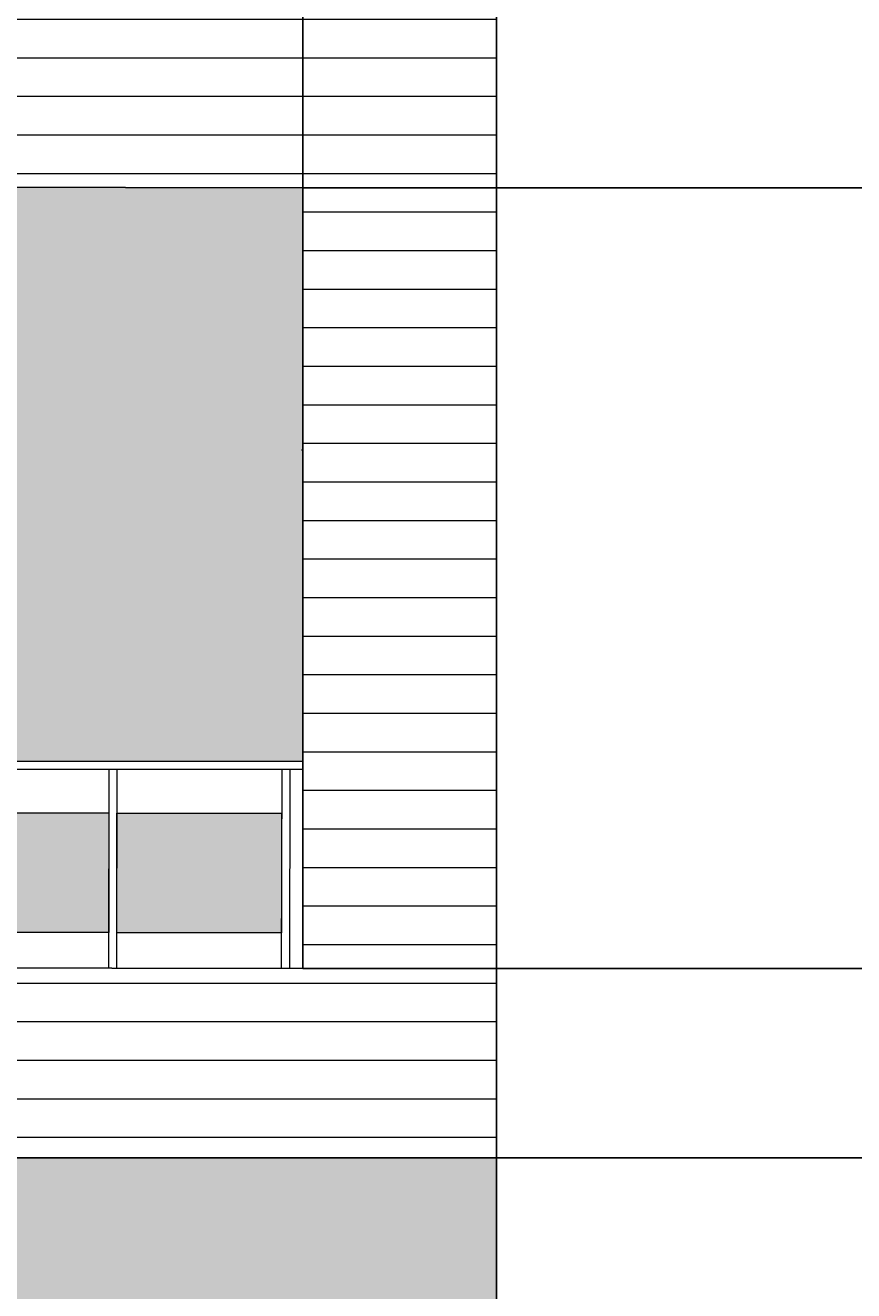
# Model space of a CAD drawing. Units: inches. Extents: x 36 to 594, y 79 to 831.
# Tile 14 of 30: x 390 to 492, y 290 to 446. Entities that reach past the tile are written whole.
import ezdxf

# ---------------------------------------------------------------- set-up
doc = ezdxf.new("R2010")
doc.units = ezdxf.units.IN
doc.header["$MEASUREMENT"] = 0
for name, color, linetype, lineweight in [('A-ANNO-DIMS', 2, 'Continuous', 18), ('A-ELEV', 7, 'Continuous', 25), ('A-ELEV-PATT', 8, 'Continuous', 13), ('A-GLAZ', 4, 'Continuous', 18)]:
    doc.layers.add(name, color=color, linetype=linetype, lineweight=lineweight)
doc.styles.get("Standard").update_dxf_attribs({"font": 'arial.ttf'})
doc.dimstyles.get("Standard").update_dxf_attribs({"dimtxt": 0.8125, "dimasz": 0.18, "dimexe": 0.18, "dimexo": 0.0625, "dimgap": 0.09, "dimtad": 0, "dimtih": 1, "dimtoh": 1, "dimdec": 4, "dimzin": 0, "dimdsep": 46, "dimlunit": 4, "dimtxsty": 'Standard', "dimcen": 0.09, "dimadec": 0, "dimazin": 0, "dimtfac": 1, "dimtdec": 4, "dimtofl": 0, "dimtmove": 0, "dimatfit": 3, "dimfxl": 1, "dimtolj": 1, "dimtzin": 0, "dimarcsym": 0})

# ---------------------------------------------------------------- blocks, each defined once
blk = doc.blocks.new('GLAZ-PANEL')
blk.add_lwpolyline([(0, 14.77), (20.28, 14.77), (20.28, 0), (0, 0)], close=True)
blk = doc.blocks.new('*D31')
at = {"layer": 'A-ANNO-DIMS', "color": 0, "lineweight": -2, "transparency": 16777216}
for p, q in [((448.45, 306.21), (592.85, 306.21)), ((592.67, 306.03), (592.67, 229.08)), ((592.67, 151.11), (592.67, 228.07)), ((401.61, 150.93), (592.85, 150.93))]:
    blk.add_line(p, q, dxfattribs=at)
at = {"layer": 'A-ANNO-DIMS', "color": 0, "transparency": 16777216}
for points in [[(592.64, 306.03), (592.7, 306.03), (592.67, 306.21)], [(592.64, 151.11), (592.7, 151.11), (592.67, 150.93)]]:
    blk.add_solid(points, dxfattribs=at)
at = {"layer": 'Defpoints', "color": 0, "transparency": 16777216}
for p in [(448.39, 306.21), (592.67, 306.21), (401.55, 150.93)]:
    blk.add_point(p, dxfattribs=at)
at = {"layer": 'A-ANNO-DIMS', "color": 0, "transparency": 16777216, "insert": (592.67, 228.57), "char_height": 0.812, "attachment_point": 5}
blk.add_mtext('\\A1;155.28', dxfattribs=at)
blk = doc.blocks.new('*D32')
at = {"layer": 'A-ANNO-DIMS', "color": 0, "lineweight": -2, "transparency": 16777216}
for p, q in [((424.61, 329.53), (592.85, 329.53)), ((592.67, 329.35), (592.67, 318.38)), ((592.67, 306.39), (592.67, 317.37)), ((448.45, 306.21), (592.85, 306.21))]:
    blk.add_line(p, q, dxfattribs=at)
at = {"layer": 'A-ANNO-DIMS', "color": 0, "transparency": 16777216}
for points in [[(592.64, 329.35), (592.7, 329.35), (592.67, 329.53)], [(592.64, 306.39), (592.7, 306.39), (592.67, 306.21)]]:
    blk.add_solid(points, dxfattribs=at)
at = {"layer": 'Defpoints', "color": 0, "transparency": 16777216}
for p in [(424.55, 329.53), (592.67, 329.53), (448.39, 306.21)]:
    blk.add_point(p, dxfattribs=at)
at = {"layer": 'A-ANNO-DIMS', "color": 0, "transparency": 16777216, "insert": (592.67, 317.87), "char_height": 0.812, "attachment_point": 5}
blk.add_mtext('\\A1;23.32', dxfattribs=at)
blk = doc.blocks.new('*D33')
at = {"layer": 'A-ANNO-DIMS', "color": 0, "lineweight": -2, "transparency": 16777216}
for p, q in [((424.61, 425.73), (592.85, 425.73)), ((592.67, 425.55), (592.67, 378.14)), ((592.67, 329.71), (592.67, 377.13)), ((424.61, 329.53), (592.85, 329.53))]:
    blk.add_line(p, q, dxfattribs=at)
at = {"layer": 'A-ANNO-DIMS', "color": 0, "transparency": 16777216}
for points in [[(592.64, 425.55), (592.7, 425.55), (592.67, 425.73)], [(592.64, 329.71), (592.7, 329.71), (592.67, 329.53)]]:
    blk.add_solid(points, dxfattribs=at)
at = {"layer": 'Defpoints', "color": 0, "transparency": 16777216}
for p in [(424.55, 425.73), (592.67, 425.73), (424.55, 329.53)]:
    blk.add_point(p, dxfattribs=at)
at = {"layer": 'A-ANNO-DIMS', "color": 0, "transparency": 16777216, "insert": (592.67, 377.63), "char_height": 0.812, "attachment_point": 5}
blk.add_mtext('\\A1;96.2', dxfattribs=at)
blk = doc.blocks.new('*D34')
at = {"layer": 'A-ANNO-DIMS', "color": 0, "lineweight": -2, "transparency": 16777216}
for p, q in [((448.45, 450.21), (592.85, 450.21)), ((592.67, 450.03), (592.67, 438.48)), ((592.67, 425.91), (592.67, 437.47)), ((424.61, 425.73), (592.85, 425.73))]:
    blk.add_line(p, q, dxfattribs=at)
at = {"layer": 'A-ANNO-DIMS', "color": 0, "transparency": 16777216}
for points in [[(592.64, 450.03), (592.7, 450.03), (592.67, 450.21)], [(592.64, 425.91), (592.7, 425.91), (592.67, 425.73)]]:
    blk.add_solid(points, dxfattribs=at)
at = {"layer": 'Defpoints', "color": 0, "transparency": 16777216}
for p in [(448.39, 450.21), (592.67, 450.21), (424.55, 425.73)]:
    blk.add_point(p, dxfattribs=at)
at = {"layer": 'A-ANNO-DIMS', "color": 0, "transparency": 16777216, "insert": (592.67, 437.97), "char_height": 0.812, "attachment_point": 5}
blk.add_mtext('\\A1;24.48', dxfattribs=at)
blk = doc.blocks.new('*D59')
at = {"layer": 'A-ANNO-DIMS', "color": 0, "lineweight": -2, "transparency": 16777216}
for p, q in [((355.86, 355.15), (355.86, 830.73)), ((356.04, 830.55), (388.74, 830.55)), ((424.37, 830.55), (391.67, 830.55)), ((424.55, 355.15), (424.55, 830.73))]:
    blk.add_line(p, q, dxfattribs=at)
at = {"layer": 'A-ANNO-DIMS', "color": 0, "transparency": 16777216}
for points in [[(356.04, 830.58), (356.04, 830.52), (355.86, 830.55)], [(424.37, 830.58), (424.37, 830.52), (424.55, 830.55)]]:
    blk.add_solid(points, dxfattribs=at)
at = {"layer": 'Defpoints', "color": 0, "transparency": 16777216}
for p in [(424.55, 830.55), (355.86, 355.08), (424.55, 355.08)]:
    blk.add_point(p, dxfattribs=at)
at = {"layer": 'A-ANNO-DIMS', "color": 0, "transparency": 16777216, "insert": (390.2, 830.55), "char_height": 0.812, "attachment_point": 5}
blk.add_mtext('\\A1;68.69', dxfattribs=at)

msp = doc.modelspace()

# ---------------------------------------------------------------- hatches: boundary and pattern name
at = {"layer": 'A-ELEV-PATT'}
h = msp.add_hatch(color=256, dxfattribs=at)
h.dxf.hatch_style = 1
h.paths.add_polyline_path([(398.0873, 796.0465), (269.3592, 796.0465), (269.3592, 770.1455), (397.8159, 770.1455)])
h.paths.add_polyline_path([(397.7518, 764.0341), (269.3592, 764.0341), (269.3592, 630.0394), (341.8367, 630.0394), (341.8367, 720.595), (335.0881, 728.3699), (329.982, 735.3373), (345.3661, 727.7743), (397.1052, 702.3389)])
h.paths.add_polyline_path([(341.8367, 594.2124), (201.4189, 594.2124), (201.4189, 475.4136), (232.8216, 475.4136), (232.8216, 524.6037), (341.8367, 524.6037)])
h.paths.add_polyline_path([(177.525, 594.2124), (118.7598, 594.2124), (118.7598, 450.2124), (177.525, 450.2124)])
h.paths.add_polyline_path([(424.4958, 594.2124), (365.7306, 594.2124), (365.7306, 450.2124), (424.4958, 450.2124)])
h.paths.add_polyline_path([(241.3553, 404.2737), (355.8569, 404.2737), (355.8569, 355.0836), (424.5492, 355.0836), (424.5492, 425.7333), (118.7598, 426.2844), (118.7598, 355.0836), (241.3553, 355.0836)])
h.paths.add_polyline_path([(448.3898, 306.2124), (217.0273, 306.2124), (217.0273, 142.2124), (254.0293, 142.2124), (254.0293, 150.9347), (254.0293, 286.1802), (401.5491, 286.1802), (401.5491, 150.9347), (401.5491, 142.2124), (448.3898, 142.2124)])
h.paths.add_polyline_path([(448.3898, 142.2124), (401.5491, 142.2124), (217.0273, 142.2124), (217.0273, 114.2124), (448.3898, 114.2124)])
h.paths.add_polyline_path([(217.0273, 306.2124), (174.7353, 306.2124), (94.8658, 306.2124), (94.8658, 162.2124), (103.3368, 162.2124), (103.3368, 264.6224), (103.3368, 286.1802), (217.0273, 286.1802)])
h = msp.add_hatch(color=256, dxfattribs=at)
h.dxf.hatch_style = 1
h.set_gradient(color1=(192, 192, 192), color2=(0, 0, 0))
h.paths.add_polyline_path([(243.19, 469.3251), (222.9132, 469.3251), (222.9132, 454.5571), (243.1634, 454.5571)])
h.paths.add_polyline_path([(264.4667, 469.2868), (244.1899, 469.2868), (244.1899, 454.5188), (264.4401, 454.5188)])
h.paths.add_polyline_path([(285.7435, 469.2484), (265.4667, 469.2484), (265.4667, 454.4804), (285.7168, 454.4804)])
h.paths.add_polyline_path([(307.0202, 469.2101), (286.7434, 469.2101), (286.7434, 454.4421), (306.9936, 454.4421)])
h.paths.add_polyline_path([(328.2969, 469.1717), (308.0201, 469.1717), (308.0201, 454.4037), (328.2703, 454.4037)])
h.paths.add_polyline_path([(341.8367, 469.1334), (329.2969, 469.1334), (329.2969, 454.3654), (341.8367, 454.3654)])
h.paths.add_polyline_path([(221.9133, 469.3635), (201.6365, 469.3635), (201.6365, 454.5955), (221.8866, 454.5955)])
h.paths.add_polyline_path([(145.3401, 349.1868), (125.0633, 349.1868), (125.0633, 334.4189), (145.3134, 334.4189)])
h.paths.add_polyline_path([(166.6168, 349.1485), (146.34, 349.1485), (146.34, 334.3805), (166.5902, 334.3805)])
h.paths.add_polyline_path([(187.8935, 349.1101), (167.6167, 349.1101), (167.6167, 334.3422), (187.8669, 334.3422)])
h.paths.add_polyline_path([(209.1703, 349.0718), (188.8935, 349.0718), (188.8935, 334.3038), (209.1436, 334.3038)])
h.paths.add_polyline_path([(230.447, 349.0335), (210.1702, 349.0335), (210.1702, 334.2655), (230.4204, 334.2655)])
h.paths.add_polyline_path([(251.7237, 348.9951), (231.4469, 348.9951), (231.4469, 334.2271), (251.6971, 334.2271)])
h.paths.add_polyline_path([(273.0005, 348.9568), (252.7236, 348.9568), (252.7236, 334.1888), (272.9738, 334.1888)])
h.paths.add_polyline_path([(294.2772, 348.9184), (274.0004, 348.9184), (274.0004, 334.1504), (294.2506, 334.1504)])
h.paths.add_polyline_path([(315.5539, 348.8801), (295.2771, 348.8801), (295.2771, 334.1121), (315.5273, 334.1121)])
h.paths.add_polyline_path([(336.8306, 348.8417), (316.5538, 348.8417), (316.5538, 334.0737), (336.804, 334.0737)])
h.paths.add_polyline_path([(358.1074, 348.8034), (337.8306, 348.8034), (337.8306, 334.0354), (358.0808, 334.0354)])
h.paths.add_polyline_path([(379.3841, 348.765), (359.1073, 348.765), (359.1073, 333.997), (379.3575, 333.997)])
h.paths.add_polyline_path([(400.6608, 348.7267), (380.384, 348.7267), (380.384, 333.9587), (400.6342, 333.9587)])
h.paths.add_polyline_path([(421.9376, 348.6883), (401.6608, 348.6883), (401.6608, 333.9204), (421.911, 333.9204)])
h.paths.add_polyline_path([(103.3368, 162.2124), (94.8658, 162.2124), (94.8658, 150.2124), (94.8658, 114.2124), (103.3368, 114.2124)])
h.paths.add_polyline_path([(217.0273, 132.2124), (103.3368, 132.2124), (103.3368, 122.2124), (217.0273, 122.2124)])
h.paths.add_polyline_path([(217.0273, 122.2124), (103.3368, 122.2124), (103.3368, 114.2124), (217.0273, 114.2124)])
h.paths.add_polyline_path([(217.0273, 142.2124), (174.7353, 142.2124), (103.3368, 142.2124), (103.3368, 132.2124), (217.0273, 132.2124)])
h.paths.add_polyline_path([(217.0273, 152.2124), (103.3368, 152.2124), (103.3368, 142.2124), (174.7353, 142.2124), (217.0273, 142.2124)])
h.paths.add_polyline_path([(217.0273, 162.2124), (103.3368, 162.2124), (103.3368, 152.2124), (217.0273, 152.2124)])
h = msp.add_hatch(dxfattribs=at)
h.set_pattern_fill('ANSI31', color=256, scale=38, angle=135)
h.paths.add_polyline_path([(448.3898, 450.2124), (94.8658, 450.2124), (94.8658, 306.2124), (174.7353, 306.2124), (448.3898, 306.2124), (448.3898, 367.5118)])
h.paths.add_polyline_path([(424.5492, 425.7333), (424.5492, 329.5325), (118.7598, 330.0836), (118.7598, 354.0836), (118.7598, 426.2844)], flags=16)
h.paths.add_polyline_path([(355.8569, 404.2737), (355.8569, 355.0836), (241.3553, 355.0836), (241.3553, 404.2737)], flags=0)
h.paths.add_polyline_path([(269.0393, 390.7924), (269.0393, 355.0836), (244.8248, 355.0836), (244.8248, 364.0887), (263.8892, 364.0887), (263.8892, 355.0836), (267.0393, 355.0836), (267.0393, 390.7924)], flags=0)
h.paths.add_polyline_path([(303.9765, 436.9126, -1), (313.1496, 436.9126, -1)], flags=16)
h.paths.add_polyline_path([(421.9473, 354.0836), (421.9376, 348.6883), (421.9376, 333.9204), (401.6342, 333.9204), (401.6705, 354.0836), (400.6705, 354.0836), (400.6608, 348.7267), (400.6608, 333.9587), (380.3574, 333.9587), (380.3937, 354.0836), (379.3937, 354.0836), (379.3841, 348.765), (379.3841, 333.997), (359.0807, 333.997), (359.1169, 354.0836), (358.1169, 354.0836), (358.1074, 348.8034), (358.1074, 334.0354), (337.804, 334.0354), (337.8401, 354.0836), (336.8401, 354.0836), (336.8306, 348.8417), (336.8306, 334.0737), (316.5272, 334.0737), (316.5633, 354.0836), (315.5633, 354.0836), (315.5539, 348.8801), (315.5539, 334.1121), (295.2505, 334.1121), (295.2865, 354.0836), (294.2865, 354.0836), (294.2772, 348.9184), (294.2772, 334.1504), (273.9738, 334.1504), (274.0097, 354.0836), (273.0097, 354.0836), (273.0005, 348.9568), (273.0005, 334.1888), (252.697, 334.1888), (252.7329, 354.0836), (251.7329, 354.0836), (251.7237, 348.9951), (251.7237, 334.2271), (231.4203, 334.2271), (231.4561, 354.0836), (230.4561, 354.0836), (230.447, 349.0335), (230.447, 334.2655), (210.1436, 334.2655), (210.1793, 354.0836), (209.1793, 354.0836), (209.1703, 349.0718), (209.1703, 334.3038), (188.8668, 334.3038), (188.9025, 354.0836), (187.9025, 354.0836), (187.8935, 349.1101), (187.8935, 334.3422), (167.5901, 334.3422), (167.6257, 354.0836), (166.6257, 354.0836), (166.6168, 349.1485), (166.6168, 334.3805), (146.3134, 334.3805), (146.3489, 354.0836), (145.3489, 354.0836), (145.3401, 349.1868), (145.3401, 334.4189), (125.0366, 334.4189), (125.0721, 354.0836)], flags=0)
h.paths.add_polyline_path([(266.285, 436.9126, -1), (275.458, 436.9126, -1)], flags=16)
h.paths.add_polyline_path([(367.0204, 316.8739, -1), (357.8474, 316.8739, -1)], flags=16)
h.paths.add_polyline_path([(347.6933, 316.8739, -1), (338.5202, 316.8739, -1)], flags=16)
h.paths.add_polyline_path([(329.574, 316.8739, -1), (320.401, 316.8739, -1)], flags=16)
h.paths.add_polyline_path([(263.8892, 385.1199), (263.8892, 368.1628), (244.8248, 368.1628), (244.8248, 385.1199)], flags=0)
h.paths.add_polyline_path([(216.2543, 436.9126, -1), (225.4274, 436.9126, -1)], flags=16)
h.paths.add_polyline_path([(275.458, 316.8739, -1), (266.285, 316.8739, -1)], flags=16)
h.paths.add_polyline_path([(225.4274, 316.8739, -1), (216.2543, 316.8739, -1)], flags=16)

# ---------------------------------------------------------------- linework, layer by layer
at = {"layer": 'A-ELEV'}
for p, q in [((448.3898, 450.2124), (448.3898, 367.5118)), ((448.3898, 142.2124), (448.3898, 367.5118)), ((174.7353, 306.2124), (448.3898, 306.2124))]:
    msp.add_line(p, q, dxfattribs=at)
msp.add_lwpolyline([(118.7598, 426.2844), (424.5492, 425.7333), (424.5492, 329.5325), (118.7598, 330.0836)], close=True, dxfattribs=at)
at = {"layer": 'A-GLAZ'}
for p, q in [((424.5492, 393.4115), (424.3898, 393.4115)), ((118.7598, 355.0836), (424.5492, 355.0836)), ((118.7598, 354.0836), (424.5492, 354.0836)), ((400.6705, 354.0836), (400.6264, 329.6139)), ((401.6705, 354.0836), (401.6264, 329.6121)), ((421.9473, 354.0836), (421.9031, 329.5756)), ((422.9473, 354.0836), (422.9031, 329.5738))]:
    msp.add_line(p, q, dxfattribs=at)

# ---------------------------------------------------------------- block references
for p in [(380.3838, 333.9588), (401.6605, 333.9205)]:
    msp.add_blockref('GLAZ-PANEL', p, dxfattribs=at)

# ---------------------------------------------------------------- dimensions: what is measured, and where the dimension line sits
at = {"layer": 'A-ANNO-DIMS'}
dim = msp.add_linear_dim(base=(424.5492, 830.5465), p1=(355.8569, 355.0836), p2=(424.5492, 355.0836), dimstyle='Standard', override={"dimdec": 2, "dimlfac": 1, "dimrnd": 0, "dimzin": 0, "dimdsep": 46, "dimlunit": 2}, dxfattribs=at)
dim.commit()
dim.dimension.update_dxf_attribs({"geometry": '*D59', "text_midpoint": (390.203, 830.5465)})
for base, p1, p2, override, picture, middle in [((592.6689, 450.2124), (424.5492, 425.7333), (448.3898, 450.2124), {"dimdec": 2, "dimlfac": 1, "dimrnd": 0, "dimzin": 0, "dimdsep": 46, "dimlunit": 2}, '*D34', (592.6689, 437.9728)), ((592.6689, 425.7333), (424.5492, 329.5325), (424.5492, 425.7333), {"dimdec": 1, "dimlfac": 1, "dimrnd": 0, "dimzin": 0, "dimdsep": 46, "dimlunit": 2}, '*D33', (592.6689, 377.6329)), ((592.6689, 329.5325), (448.3898, 306.2124), (424.5492, 329.5325), {"dimdec": 2, "dimlfac": 1, "dimrnd": 0, "dimzin": 0, "dimdsep": 46, "dimlunit": 2}, '*D32', (592.6689, 317.8724)), ((592.6689, 306.2124), (401.5491, 150.9347), (448.3898, 306.2124), {"dimdec": 2, "dimlfac": 1, "dimrnd": 0, "dimzin": 0, "dimdsep": 46, "dimlunit": 2}, '*D31', (592.6689, 228.5735))]:
    dim = msp.add_linear_dim(base=base, p1=p1, p2=p2, angle=90, dimstyle='Standard', override=override, dxfattribs=at)
    dim.commit()
    dim.dimension.update_dxf_attribs({"geometry": picture, "text_midpoint": middle})

doc.saveas('drawing.dxf')
